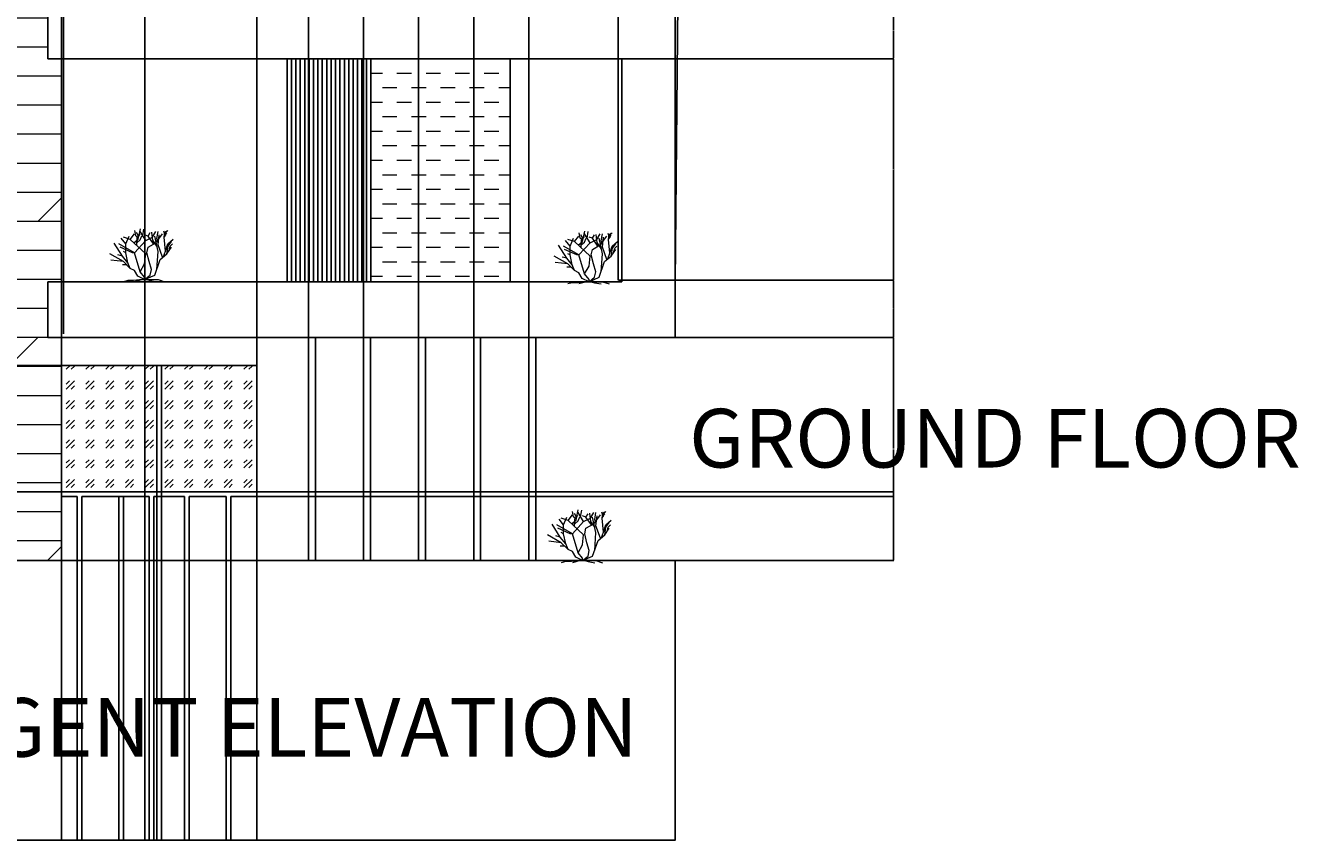
# Model space of a CAD drawing. Units: inches. Extents: x 250 to 1217, y -42 to 832.
# Tile 5 of 7: x 670 to 1217, y -42 to 309. Entities that reach past the tile are written whole.
import ezdxf

# ---------------------------------------------------------------- set-up
doc = ezdxf.new("R2010")
doc.units = ezdxf.units.IN
doc.header["$MEASUREMENT"] = 0
for name, color, linetype, lineweight in [('A-ANNO-DIMS', 2, 'Continuous', 18), ('A-ANNO-TEXT', 7, 'Continuous', 25), ('A-ELEV', 7, 'Continuous', 25), ('A-ELEV-PATT', 8, 'Continuous', 13), ('L-PLNT', 3, 'Continuous', 13)]:
    doc.layers.add(name, color=color, linetype=linetype, lineweight=lineweight)
doc.styles.get("Standard").update_dxf_attribs({"font": 'arial.ttf'})
doc.dimstyles.get("Standard").update_dxf_attribs({"dimtxt": 0.18, "dimasz": 0.18, "dimexe": 0.18, "dimexo": 0.0625, "dimgap": 0.09, "dimtad": 0, "dimtih": 1, "dimtoh": 1, "dimdec": 4, "dimzin": 0, "dimdsep": 46, "dimtxsty": 'Standard', "dimcen": 0.09, "dimadec": 0, "dimazin": 0, "dimtfac": 1, "dimtdec": 4, "dimtofl": 0, "dimtmove": 0, "dimatfit": 3, "dimfxl": 1, "dimtolj": 1, "dimtzin": 0, "dimarcsym": 0})

# ---------------------------------------------------------------- blocks, each defined once
blk = doc.blocks.new('*U2')
for p, q in [((-12.471, 19.775), (-12.898, 22.044)), ((-11.433, 18.289), (-10.457, 22.749)), ((-9.48, 19.775), (-8.992, 22.592)), ((0.041, 20.714), (1.384, 22.044)), ((-18.24, 11.04), (-21.755, 16.655)), ((-16.8, 16.32), (-18.72, 18.72)), ((-14.88, 18.24), (-17.76, 19.2)), ((-16.8, 16.32), (-15.36, 19.68)), ((-14.88, 18.24), (-12.96, 20.64)), ((-8.16, 12), (-14.88, 18.24)), ((-13.325, 16.724), (-11.433, 18.289)), ((-12.96, 12.48), (-8.16, 17.76)), ((-11.677, 19.071), (-12.471, 19.775)), ((-11.28, 19.619), (-12.104, 21.184)), ((-12.043, 15.628), (-11.921, 18.836)), ((-11.982, 16.802), (-10.579, 18.054)), ((-11.921, 18.836), (-10.64, 20.401)), ((-10.579, 18.054), (-9.846, 19.697)), ((-8.16, 17.76), (-10.56, 21.6)), ((-7.2, 19.68), (-8.64, 20.16)), ((-8.16, 17.76), (-5.28, 19.2)), ((-7.2, 19.68), (-6.24, 21.12)), ((-4.8, 16.32), (-7.2, 19.68)), ((-7.2, 14.88), (-3.84, 16.8)), ((-5.086, 17.741), (-5.513, 21.34)), ((-5.28, 19.2), (-3.84, 21.6)), ((-3.377, 15.315), (-5.086, 17.819)), ((-2.88, 12.96), (-4.32, 19.68)), ((-3.84, 16.8), (-0.96, 20.64)), ((-3.377, 18.602), (-2.888, 21.575)), ((-2.766, 16.802), (-3.377, 18.602)), ((-2.88, 15.84), (-2.4, 20.16)), ((-0.508, 21.888), (-0.081, 20.558)), ((-0.203, 19.149), (0.102, 21.34)), ((0.346, 13.203), (-0.203, 19.149)), ((-0.142, 19.384), (0.59, 20.401)), ((-0.02, 20.01), (0.896, 21.105)), ((0.102, 21.34), (0.835, 21.888)), ((1.323, 16.254), (3.642, 18.289)), ((1.44, 15.36), (2.88, 17.28)), ((-17.76, 8.64), (-23.663, 11.961)), ((-18.24, 11.04), (-20.16, 11.52)), ((-12.96, 12.48), (-19.68, 16.32)), ((-13.92, 12.48), (-19.2, 14.88)), ((-15.84, 8.16), (-18.24, 11.04)), ((-16.8, 12.48), (-17.76, 12.96)), ((-16.8, 12.48), (-16.8, 16.32)), ((-15.84, 8.16), (-16.8, 12.48)), ((-12.96, 12.48), (-13.92, 12.48)), ((-10.56, 4.32), (-12.96, 12.48)), ((-8.64, 7.68), (-8.16, 12)), ((-7.68, 12.48), (-7.2, 14.88)), ((-6.72, 8.64), (-7.68, 12.48)), ((-3.36, 5.28), (-2.88, 12.96)), ((-0.96, 10.56), (-2.88, 15.84)), ((-1.92, 9.6), (0.96, 12)), ((-0.48, 10.8), (0.346, 13.203)), ((0.346, 13.203), (1.323, 16.254)), ((0.96, 12), (1.44, 15.36)), ((0.96, 12), (2.88, 14.88)), ((1.92, 13.44), (2.4, 15.36)), ((2.4, 15.36), (3.36, 16.32)), ((-17.76, 8.64), (-23.128, 9.222)), ((-16.32, 7.2), (-18.24, 7.2)), ((-14.88, 5.76), (-17.76, 8.64)), ((-14.88, 5.76), (-15.84, 8.16)), ((-12.96, 4.8), (-14.88, 5.76)), ((-10.56, 4.32), (-8.64, 7.68)), ((-5.76, 5.28), (-6.72, 8.64)), ((-4.32, 2.88), (-1.92, 9.6)), ((-15.84, 0.48), (-17.76, 0)), ((-13.44, 0.48), (-15.84, 0.48)), ((-9.6, 0.96), (-13.44, 0.48)), ((-11.52, 2.4), (-12.96, 4.8)), ((-9.6, 0.96), (-12.96, 0)), ((-8.64, 0.96), (-11.52, 2.4)), ((-8.64, 1.92), (-10.56, 4.32)), ((-9.6, 0.96), (-7.68, 0.96)), ((-8.64, 0.96), (-4.32, 2.88)), ((-8.64, 0.96), (-6.24, 2.88)), ((-8.64, 0.96), (-8.64, 1.92)), ((-8.64, 0.96), (-2.88, 0.96)), ((-7.68, 0.96), (-6.24, 0.48)), ((-6.24, 2.88), (-5.76, 5.28)), ((-6.24, 0.48), (-3.36, 0)), ((-2.88, 0.96), (0, 0))]:
    blk.add_line(p, q)
blk = doc.blocks.new('*D7')
at = {"layer": 'A-ANNO-DIMS', "color": 0, "lineweight": -2, "transparency": 16777216}
for p, q in [((347.9, 78), (347.9, -41.6)), ((948.98, 78.86), (948.98, -41.6)), ((348.08, -41.42), (648.06, -41.42)), ((948.8, -41.42), (648.82, -41.42))]:
    blk.add_line(p, q, dxfattribs=at)
at = {"layer": 'A-ANNO-DIMS', "color": 0, "transparency": 16777216}
for points in [[(348.08, -41.39), (348.08, -41.45), (347.9, -41.42)], [(948.8, -41.39), (948.8, -41.45), (948.98, -41.42)]]:
    blk.add_solid(points, dxfattribs=at)
at = {"layer": 'Defpoints', "color": 0, "transparency": 16777216}
for p in [(347.9, 78.06), (948.98, 78.93), (948.98, -41.42)]:
    blk.add_point(p, dxfattribs=at)
at = {"layer": 'A-ANNO-DIMS', "color": 0, "transparency": 16777216, "insert": (648.44, -41.42), "char_height": 0.18, "attachment_point": 5}
blk.add_mtext('\\A1;601.1', dxfattribs=at)
blk = doc.blocks.new('*D12')
at = {"layer": 'A-ANNO-DIMS', "color": 0, "lineweight": -2, "transparency": 16777216}
for p, q in [((949.05, 174.93), (1043.08, 174.93)), ((1042.9, 174.75), (1042.9, 127.11)), ((1042.9, 79.11), (1042.9, 126.75)), ((949.05, 78.93), (1043.08, 78.93))]:
    blk.add_line(p, q, dxfattribs=at)
at = {"layer": 'A-ANNO-DIMS', "color": 0, "transparency": 16777216}
for points in [[(1042.87, 174.75), (1042.93, 174.75), (1042.9, 174.93)], [(1042.87, 79.11), (1042.93, 79.11), (1042.9, 78.93)]]:
    blk.add_solid(points, dxfattribs=at)
at = {"layer": 'Defpoints', "color": 0, "transparency": 16777216}
for p in [(948.98, 174.93), (1042.9, 174.93), (948.98, 78.93)]:
    blk.add_point(p, dxfattribs=at)
at = {"layer": 'A-ANNO-DIMS', "color": 0, "transparency": 16777216, "insert": (1042.9, 126.93), "char_height": 0.18, "attachment_point": 5}
blk.add_mtext('\\A1;96', dxfattribs=at)
blk = doc.blocks.new('*D13')
at = {"layer": 'A-ANNO-DIMS', "color": 0, "lineweight": -2, "transparency": 16777216}
for p, q in [((924.56, 199.59), (1043.08, 199.59)), ((1042.9, 199.41), (1042.9, 187.44)), ((1042.9, 175.11), (1042.9, 187.08)), ((949.05, 174.93), (1043.08, 174.93))]:
    blk.add_line(p, q, dxfattribs=at)
at = {"layer": 'A-ANNO-DIMS', "color": 0, "transparency": 16777216}
for points in [[(1042.87, 199.41), (1042.93, 199.41), (1042.9, 199.59)], [(1042.87, 175.11), (1042.93, 175.11), (1042.9, 174.93)]]:
    blk.add_solid(points, dxfattribs=at)
at = {"layer": 'Defpoints', "color": 0, "transparency": 16777216}
for p in [(924.49, 199.59), (1042.9, 199.59), (948.98, 174.93)]:
    blk.add_point(p, dxfattribs=at)
at = {"layer": 'A-ANNO-DIMS', "color": 0, "transparency": 16777216, "insert": (1042.9, 187.26), "char_height": 0.18, "attachment_point": 5}
blk.add_mtext('\\A1;24.665', dxfattribs=at)
blk = doc.blocks.new('*D14')
at = {"layer": 'A-ANNO-DIMS', "color": 0, "lineweight": -2, "transparency": 16777216}
for p, q in [((926.12, 294.93), (1043.08, 294.93)), ((1042.9, 294.75), (1042.9, 247.44)), ((1042.9, 199.77), (1042.9, 247.08)), ((924.56, 199.59), (1043.08, 199.59))]:
    blk.add_line(p, q, dxfattribs=at)
at = {"layer": 'A-ANNO-DIMS', "color": 0, "transparency": 16777216}
for points in [[(1042.87, 294.75), (1042.93, 294.75), (1042.9, 294.93)], [(1042.87, 199.77), (1042.93, 199.77), (1042.9, 199.59)]]:
    blk.add_solid(points, dxfattribs=at)
at = {"layer": 'Defpoints', "color": 0, "transparency": 16777216}
for p in [(926.06, 294.93), (1042.9, 294.93), (924.49, 199.59)]:
    blk.add_point(p, dxfattribs=at)
at = {"layer": 'A-ANNO-DIMS', "color": 0, "transparency": 16777216, "insert": (1042.9, 247.26), "char_height": 0.18, "attachment_point": 5}
blk.add_mtext('\\A1;95.34', dxfattribs=at)
blk = doc.blocks.new('*D15')
at = {"layer": 'A-ANNO-DIMS', "color": 0, "lineweight": -2, "transparency": 16777216}
for p, q in [((950.12, 318.93), (1043.08, 318.93)), ((1042.9, 318.75), (1042.9, 307.11)), ((1042.9, 295.11), (1042.9, 306.75)), ((926.12, 294.93), (1043.08, 294.93))]:
    blk.add_line(p, q, dxfattribs=at)
at = {"layer": 'A-ANNO-DIMS', "color": 0, "transparency": 16777216}
for points in [[(1042.87, 318.75), (1042.93, 318.75), (1042.9, 318.93)], [(1042.87, 295.11), (1042.93, 295.11), (1042.9, 294.93)]]:
    blk.add_solid(points, dxfattribs=at)
at = {"layer": 'Defpoints', "color": 0, "transparency": 16777216}
for p in [(950.06, 318.93), (1042.9, 318.93), (926.06, 294.93)]:
    blk.add_point(p, dxfattribs=at)
at = {"layer": 'A-ANNO-DIMS', "color": 0, "transparency": 16777216, "insert": (1042.9, 306.93), "char_height": 0.18, "attachment_point": 5}
blk.add_mtext('\\A1;24', dxfattribs=at)
blk = doc.blocks.new('*D27')
at = {"layer": 'A-ANNO-DIMS', "color": 0, "lineweight": -2, "transparency": 16777216}
for p, q in [((624.98, 174.99), (624.98, 831.77)), ((625.16, 831.59), (655.07, 831.59)), ((685.76, 831.59), (655.86, 831.59)), ((685.94, 176.49), (685.94, 831.77))]:
    blk.add_line(p, q, dxfattribs=at)
at = {"layer": 'A-ANNO-DIMS', "color": 0, "transparency": 16777216}
for points in [[(625.16, 831.62), (625.16, 831.56), (624.98, 831.59)], [(685.76, 831.62), (685.76, 831.56), (685.94, 831.59)]]:
    blk.add_solid(points, dxfattribs=at)
at = {"layer": 'Defpoints', "color": 0, "transparency": 16777216}
for p in [(685.94, 831.59), (685.94, 176.43), (624.98, 174.93)]:
    blk.add_point(p, dxfattribs=at)
at = {"layer": 'A-ANNO-DIMS', "color": 0, "transparency": 16777216, "insert": (655.46, 831.59), "char_height": 0.18, "attachment_point": 5}
blk.add_mtext('\\A1;60.96', dxfattribs=at)
blk = doc.blocks.new('*D28')
at = {"layer": 'A-ANNO-DIMS', "color": 0, "lineweight": -2, "transparency": 16777216}
for p, q in [((685.94, 176.49), (685.94, 831.77)), ((686.12, 831.59), (727.07, 831.59)), ((768.8, 831.59), (727.86, 831.59)), ((768.98, 162.99), (768.98, 831.77))]:
    blk.add_line(p, q, dxfattribs=at)
at = {"layer": 'A-ANNO-DIMS', "color": 0, "transparency": 16777216}
for points in [[(686.12, 831.62), (686.12, 831.56), (685.94, 831.59)], [(768.8, 831.62), (768.8, 831.56), (768.98, 831.59)]]:
    blk.add_solid(points, dxfattribs=at)
at = {"layer": 'Defpoints', "color": 0, "transparency": 16777216}
for p in [(768.98, 831.59), (685.94, 176.43), (768.98, 162.93)]:
    blk.add_point(p, dxfattribs=at)
at = {"layer": 'A-ANNO-DIMS', "color": 0, "transparency": 16777216, "insert": (727.46, 831.59), "char_height": 0.18, "attachment_point": 5}
blk.add_mtext('\\A1;83.04', dxfattribs=at)
blk = doc.blocks.new('*D29')
at = {"layer": 'A-ANNO-DIMS', "color": 0, "lineweight": -2, "transparency": 16777216}
for p, q in [((768.98, 162.99), (768.98, 831.77)), ((769.16, 831.59), (779.67, 831.59)), ((791.11, 831.59), (780.6, 831.59)), ((791.29, 174.99), (791.29, 831.77))]:
    blk.add_line(p, q, dxfattribs=at)
at = {"layer": 'A-ANNO-DIMS', "color": 0, "transparency": 16777216}
for points in [[(769.16, 831.62), (769.16, 831.56), (768.98, 831.59)], [(791.11, 831.62), (791.11, 831.56), (791.29, 831.59)]]:
    blk.add_solid(points, dxfattribs=at)
at = {"layer": 'Defpoints', "color": 0, "transparency": 16777216}
for p in [(791.29, 831.59), (791.29, 174.93), (768.98, 162.93)]:
    blk.add_point(p, dxfattribs=at)
at = {"layer": 'A-ANNO-DIMS', "color": 0, "transparency": 16777216, "insert": (780.13, 831.59), "char_height": 0.18, "attachment_point": 5}
blk.add_mtext('\\A1;22.303', dxfattribs=at)
blk = doc.blocks.new('*D30')
at = {"layer": 'A-ANNO-DIMS', "color": 0, "lineweight": -2, "transparency": 16777216}
for p, q in [((814.96, 174.99), (814.96, 831.77)), ((815.14, 831.59), (826.33, 831.59)), ((838.45, 831.59), (827.26, 831.59)), ((838.63, 174.99), (838.63, 831.77))]:
    blk.add_line(p, q, dxfattribs=at)
at = {"layer": 'A-ANNO-DIMS', "color": 0, "transparency": 16777216}
for points in [[(815.14, 831.62), (815.14, 831.56), (814.96, 831.59)], [(838.45, 831.62), (838.45, 831.56), (838.63, 831.59)]]:
    blk.add_solid(points, dxfattribs=at)
at = {"layer": 'Defpoints', "color": 0, "transparency": 16777216}
for p in [(838.63, 831.59), (814.96, 174.93), (838.63, 174.93)]:
    blk.add_point(p, dxfattribs=at)
at = {"layer": 'A-ANNO-DIMS', "color": 0, "transparency": 16777216, "insert": (826.8, 831.59), "char_height": 0.18, "attachment_point": 5}
blk.add_mtext('\\A1;23.674', dxfattribs=at)
blk = doc.blocks.new('*D31')
at = {"layer": 'A-ANNO-DIMS', "color": 0, "lineweight": -2, "transparency": 16777216}
for p, q in [((862.31, 174.99), (862.31, 831.77)), ((862.49, 831.59), (873.68, 831.59)), ((885.8, 831.59), (874.61, 831.59)), ((885.98, 174.99), (885.98, 831.77))]:
    blk.add_line(p, q, dxfattribs=at)
at = {"layer": 'A-ANNO-DIMS', "color": 0, "transparency": 16777216}
for points in [[(862.49, 831.62), (862.49, 831.56), (862.31, 831.59)], [(885.8, 831.62), (885.8, 831.56), (885.98, 831.59)]]:
    blk.add_solid(points, dxfattribs=at)
at = {"layer": 'Defpoints', "color": 0, "transparency": 16777216}
for p in [(885.98, 831.59), (862.31, 174.93), (885.98, 174.93)]:
    blk.add_point(p, dxfattribs=at)
at = {"layer": 'A-ANNO-DIMS', "color": 0, "transparency": 16777216, "insert": (874.15, 831.59), "char_height": 0.18, "attachment_point": 5}
blk.add_mtext('\\A1;23.674', dxfattribs=at)
blk = doc.blocks.new('*D32')
at = {"layer": 'A-ANNO-DIMS', "color": 0, "lineweight": -2, "transparency": 16777216}
for p, q in [((885.98, 174.99), (885.98, 831.77)), ((886.16, 831.59), (917.26, 831.59)), ((948.8, 831.59), (917.7, 831.59)), ((948.98, 174.99), (948.98, 831.77))]:
    blk.add_line(p, q, dxfattribs=at)
at = {"layer": 'A-ANNO-DIMS', "color": 0, "transparency": 16777216}
for points in [[(886.16, 831.62), (886.16, 831.56), (885.98, 831.59)], [(948.8, 831.62), (948.8, 831.56), (948.98, 831.59)]]:
    blk.add_solid(points, dxfattribs=at)
at = {"layer": 'Defpoints', "color": 0, "transparency": 16777216}
for p in [(948.98, 831.59), (885.98, 174.93), (948.98, 174.93)]:
    blk.add_point(p, dxfattribs=at)
at = {"layer": 'A-ANNO-DIMS', "color": 0, "transparency": 16777216, "insert": (917.48, 831.59), "char_height": 0.18, "attachment_point": 5}
blk.add_mtext('\\A1;63', dxfattribs=at)
blk = doc.blocks.new('*D36')
at = {"layer": 'A-ANNO-DIMS', "color": 0, "lineweight": -2, "transparency": 16777216}
for p, q in [((768.92, 162.93), (250.36, 162.93)), ((250.54, 162.75), (250.54, 135.88)), ((250.54, 108.65), (250.54, 135.51)), ((768.92, 108.47), (250.36, 108.47))]:
    blk.add_line(p, q, dxfattribs=at)
at = {"layer": 'A-ANNO-DIMS', "color": 0, "transparency": 16777216}
for points in [[(250.51, 162.75), (250.57, 162.75), (250.54, 162.93)], [(250.51, 108.65), (250.57, 108.65), (250.54, 108.47)]]:
    blk.add_solid(points, dxfattribs=at)
at = {"layer": 'Defpoints', "color": 0, "transparency": 16777216}
for p in [(250.54, 162.93), (768.98, 162.93), (768.98, 108.47)]:
    blk.add_point(p, dxfattribs=at)
at = {"layer": 'A-ANNO-DIMS', "color": 0, "transparency": 16777216, "insert": (250.54, 135.7), "char_height": 0.18, "attachment_point": 5}
blk.add_mtext('\\A1;54.46', dxfattribs=at)
blk = doc.blocks.new('*D52')
at = {"layer": 'A-ANNO-DIMS', "color": 0, "lineweight": -2, "transparency": 16777216}
for p, q in [((924.49, 199.65), (924.49, 831.77)), ((924.67, 831.59), (936.34, 831.59)), ((948.8, 831.59), (937.13, 831.59)), ((948.98, 198.99), (948.98, 831.77))]:
    blk.add_line(p, q, dxfattribs=at)
at = {"layer": 'A-ANNO-DIMS', "color": 0, "transparency": 16777216}
for points in [[(924.67, 831.62), (924.67, 831.56), (924.49, 831.59)], [(948.8, 831.62), (948.8, 831.56), (948.98, 831.59)]]:
    blk.add_solid(points, dxfattribs=at)
at = {"layer": 'Defpoints', "color": 0, "transparency": 16777216}
for p in [(948.98, 831.59), (924.49, 199.59), (948.98, 198.93)]:
    blk.add_point(p, dxfattribs=at)
at = {"layer": 'A-ANNO-DIMS', "color": 0, "transparency": 16777216, "insert": (936.74, 831.59), "char_height": 0.18, "attachment_point": 5}
blk.add_mtext('\\A1;24.49', dxfattribs=at)
blk = doc.blocks.new('*D65')
at = {"layer": 'A-ANNO-DIMS', "color": 0, "lineweight": -2, "transparency": 16777216}
for p, q in [((684.98, 78.86), (684.98, -41.6)), ((691.76, 78.86), (691.76, -41.6)), ((685.16, -41.42), (687.98, -41.42)), ((691.58, -41.42), (688.76, -41.42))]:
    blk.add_line(p, q, dxfattribs=at)
at = {"layer": 'A-ANNO-DIMS', "color": 0, "transparency": 16777216}
for points in [[(685.16, -41.39), (685.16, -41.45), (684.98, -41.42)], [(691.58, -41.39), (691.58, -41.45), (691.76, -41.42)]]:
    blk.add_solid(points, dxfattribs=at)
at = {"layer": 'Defpoints', "color": 0, "transparency": 16777216}
for p in [(684.98, 78.93), (691.76, 78.93), (691.76, -41.42)]:
    blk.add_point(p, dxfattribs=at)
at = {"layer": 'A-ANNO-DIMS', "color": 0, "transparency": 16777216, "insert": (688.37, -41.42), "char_height": 0.18, "attachment_point": 5}
blk.add_mtext('\\A1;6.774', dxfattribs=at)
blk = doc.blocks.new('*D66')
at = {"layer": 'A-ANNO-DIMS', "color": 0, "lineweight": -2, "transparency": 16777216}
for p, q in [((693.76, 78.86), (693.76, -41.6)), ((709.68, 78.86), (709.68, -41.6)), ((693.94, -41.42), (701.26, -41.42)), ((709.5, -41.42), (702.18, -41.42))]:
    blk.add_line(p, q, dxfattribs=at)
at = {"layer": 'A-ANNO-DIMS', "color": 0, "transparency": 16777216}
for points in [[(693.94, -41.39), (693.94, -41.45), (693.76, -41.42)], [(709.5, -41.39), (709.5, -41.45), (709.68, -41.42)]]:
    blk.add_solid(points, dxfattribs=at)
at = {"layer": 'Defpoints', "color": 0, "transparency": 16777216}
for p in [(693.76, 78.93), (709.68, 78.93), (709.68, -41.42)]:
    blk.add_point(p, dxfattribs=at)
at = {"layer": 'A-ANNO-DIMS', "color": 0, "transparency": 16777216, "insert": (701.72, -41.42), "char_height": 0.18, "attachment_point": 5}
blk.add_mtext('\\A1;15.928', dxfattribs=at)
blk = doc.blocks.new('*D67')
at = {"layer": 'A-ANNO-DIMS', "color": 0, "lineweight": -2, "transparency": 16777216}
for p, q in [((711.68, 78.86), (711.68, -41.6)), ((722.76, 78.86), (722.76, -41.6)), ((711.86, -41.42), (716.77, -41.42)), ((722.58, -41.42), (717.67, -41.42))]:
    blk.add_line(p, q, dxfattribs=at)
at = {"layer": 'A-ANNO-DIMS', "color": 0, "transparency": 16777216}
for points in [[(711.86, -41.39), (711.86, -41.45), (711.68, -41.42)], [(722.58, -41.39), (722.58, -41.45), (722.76, -41.42)]]:
    blk.add_solid(points, dxfattribs=at)
at = {"layer": 'Defpoints', "color": 0, "transparency": 16777216}
for p in [(711.68, 78.93), (722.76, 78.93), (722.76, -41.42)]:
    blk.add_point(p, dxfattribs=at)
at = {"layer": 'A-ANNO-DIMS', "color": 0, "transparency": 16777216, "insert": (717.22, -41.42), "char_height": 0.18, "attachment_point": 5}
blk.add_mtext('\\A1;11.072', dxfattribs=at)
blk = doc.blocks.new('*D68')
at = {"layer": 'A-ANNO-DIMS', "color": 0, "lineweight": -2, "transparency": 16777216}
for p, q in [((724.76, 78.86), (724.76, -41.6)), ((737.98, 78.86), (737.98, -41.6)), ((724.94, -41.42), (730.91, -41.42)), ((737.8, -41.42), (731.82, -41.42))]:
    blk.add_line(p, q, dxfattribs=at)
at = {"layer": 'A-ANNO-DIMS', "color": 0, "transparency": 16777216}
for points in [[(724.94, -41.39), (724.94, -41.45), (724.76, -41.42)], [(737.8, -41.39), (737.8, -41.45), (737.98, -41.42)]]:
    blk.add_solid(points, dxfattribs=at)
at = {"layer": 'Defpoints', "color": 0, "transparency": 16777216}
for p in [(724.76, 78.93), (737.98, 78.93), (737.98, -41.42)]:
    blk.add_point(p, dxfattribs=at)
at = {"layer": 'A-ANNO-DIMS', "color": 0, "transparency": 16777216, "insert": (731.37, -41.42), "char_height": 0.18, "attachment_point": 5}
blk.add_mtext('\\A1;13.226', dxfattribs=at)
blk = doc.blocks.new('*D69')
at = {"layer": 'A-ANNO-DIMS', "color": 0, "lineweight": -2, "transparency": 16777216}
for p, q in [((739.98, 78.86), (739.98, -41.6)), ((755.91, 78.86), (755.91, -41.6)), ((740.16, -41.42), (747.49, -41.42)), ((755.73, -41.42), (748.4, -41.42))]:
    blk.add_line(p, q, dxfattribs=at)
at = {"layer": 'A-ANNO-DIMS', "color": 0, "transparency": 16777216}
for points in [[(740.16, -41.39), (740.16, -41.45), (739.98, -41.42)], [(755.73, -41.39), (755.73, -41.45), (755.91, -41.42)]]:
    blk.add_solid(points, dxfattribs=at)
at = {"layer": 'Defpoints', "color": 0, "transparency": 16777216}
for p in [(739.98, 78.93), (755.91, 78.93), (755.91, -41.42)]:
    blk.add_point(p, dxfattribs=at)
at = {"layer": 'A-ANNO-DIMS', "color": 0, "transparency": 16777216, "insert": (747.95, -41.42), "char_height": 0.18, "attachment_point": 5}
blk.add_mtext('\\A1;15.928', dxfattribs=at)
blk = doc.blocks.new('*D70')
at = {"layer": 'A-ANNO-DIMS', "color": 0, "lineweight": -2, "transparency": 16777216}
for p, q in [((757.91, 78.86), (757.91, -41.6)), ((768.98, 78.86), (768.98, -41.6)), ((758.09, -41.42), (762.99, -41.42)), ((768.8, -41.42), (763.9, -41.42))]:
    blk.add_line(p, q, dxfattribs=at)
at = {"layer": 'A-ANNO-DIMS', "color": 0, "transparency": 16777216}
for points in [[(758.09, -41.39), (758.09, -41.45), (757.91, -41.42)], [(768.8, -41.39), (768.8, -41.45), (768.98, -41.42)]]:
    blk.add_solid(points, dxfattribs=at)
at = {"layer": 'Defpoints', "color": 0, "transparency": 16777216}
for p in [(757.91, 78.93), (768.98, 78.93), (768.98, -41.42)]:
    blk.add_point(p, dxfattribs=at)
at = {"layer": 'A-ANNO-DIMS', "color": 0, "transparency": 16777216, "insert": (763.45, -41.42), "char_height": 0.18, "attachment_point": 5}
blk.add_mtext('\\A1;11.072', dxfattribs=at)
blk = doc.blocks.new('*D75')
at = {"layer": 'A-ANNO-DIMS', "color": 0, "lineweight": -2, "transparency": 16777216}
for p, q in [((684.98, 108.4), (684.98, -41.6)), ((725.98, 108.4), (725.98, -41.6)), ((685.16, -41.42), (705.09, -41.42)), ((725.8, -41.42), (705.88, -41.42))]:
    blk.add_line(p, q, dxfattribs=at)
at = {"layer": 'A-ANNO-DIMS', "color": 0, "transparency": 16777216}
for points in [[(685.16, -41.39), (685.16, -41.45), (684.98, -41.42)], [(725.8, -41.39), (725.8, -41.45), (725.98, -41.42)]]:
    blk.add_solid(points, dxfattribs=at)
at = {"layer": 'Defpoints', "color": 0, "transparency": 16777216}
for p in [(684.98, 108.47), (725.98, 108.47), (725.98, -41.42)]:
    blk.add_point(p, dxfattribs=at)
at = {"layer": 'A-ANNO-DIMS', "color": 0, "transparency": 16777216, "insert": (705.48, -41.42), "char_height": 0.18, "attachment_point": 5}
blk.add_mtext('\\A1;41.00', dxfattribs=at)
blk = doc.blocks.new('*D76')
at = {"layer": 'A-ANNO-DIMS', "color": 0, "lineweight": -2, "transparency": 16777216}
for p, q in [((727.98, 108.4), (727.98, -41.6)), ((768.98, 108.4), (768.98, -41.6)), ((728.16, -41.42), (748.09, -41.42)), ((768.8, -41.42), (748.88, -41.42))]:
    blk.add_line(p, q, dxfattribs=at)
at = {"layer": 'A-ANNO-DIMS', "color": 0, "transparency": 16777216}
for points in [[(728.16, -41.39), (728.16, -41.45), (727.98, -41.42)], [(768.8, -41.39), (768.8, -41.45), (768.98, -41.42)]]:
    blk.add_solid(points, dxfattribs=at)
at = {"layer": 'Defpoints', "color": 0, "transparency": 16777216}
for p in [(727.98, 108.47), (768.98, 108.47), (768.98, -41.42)]:
    blk.add_point(p, dxfattribs=at)
at = {"layer": 'A-ANNO-DIMS', "color": 0, "transparency": 16777216, "insert": (748.48, -41.42), "char_height": 0.18, "attachment_point": 5}
blk.add_mtext('\\A1;41.00', dxfattribs=at)
blk = doc.blocks.new('*D77')
at = {"layer": 'A-ANNO-DIMS', "color": 0, "lineweight": -2, "transparency": 16777216}
for p, q in [((769.05, 108.47), (1043.08, 108.47)), ((769.05, 106.47), (1043.08, 106.47)), ((1042.9, 108.29), (1042.9, 107.65)), ((1042.9, 106.65), (1042.9, 107.28))]:
    blk.add_line(p, q, dxfattribs=at)
at = {"layer": 'A-ANNO-DIMS', "color": 0, "transparency": 16777216}
for points in [[(1042.87, 108.29), (1042.93, 108.29), (1042.9, 108.47)], [(1042.87, 106.65), (1042.93, 106.65), (1042.9, 106.47)]]:
    blk.add_solid(points, dxfattribs=at)
at = {"layer": 'Defpoints', "color": 0, "transparency": 16777216}
for p in [(768.98, 108.47), (768.98, 106.47), (1042.9, 108.47)]:
    blk.add_point(p, dxfattribs=at)
at = {"layer": 'A-ANNO-DIMS', "color": 0, "transparency": 16777216, "insert": (1042.9, 107.47), "char_height": 0.18, "attachment_point": 5}
blk.add_mtext('\\A1;2.00', dxfattribs=at)
blk = doc.blocks.new('*D98')
at = {"layer": 'A-ANNO-DIMS', "color": 0, "lineweight": -2, "transparency": 16777216}
for p, q in [((685.06, 582.86), (685.06, -41.6)), ((720.87, 583.82), (720.87, -41.6)), ((685.24, -41.42), (702.59, -41.42)), ((720.69, -41.42), (703.34, -41.42))]:
    blk.add_line(p, q, dxfattribs=at)
at = {"layer": 'A-ANNO-DIMS', "color": 0, "transparency": 16777216}
for points in [[(685.24, -41.39), (685.24, -41.45), (685.06, -41.42)], [(720.69, -41.39), (720.69, -41.45), (720.87, -41.42)]]:
    blk.add_solid(points, dxfattribs=at)
at = {"layer": 'Defpoints', "color": 0, "transparency": 16777216}
for p in [(685.06, 582.93), (720.87, 583.89), (720.87, -41.42)]:
    blk.add_point(p, dxfattribs=at)
at = {"layer": 'A-ANNO-DIMS', "color": 0, "transparency": 16777216, "insert": (702.97, -41.42), "char_height": 0.18, "attachment_point": 5}
blk.add_mtext('\\A1;35.81', dxfattribs=at)

msp = doc.modelspace()

# ---------------------------------------------------------------- hatches: boundary and pattern name
at = {"layer": 'A-ELEV-PATT'}
h = msp.add_hatch(dxfattribs=at)
h.set_pattern_fill('DOLMIT', color=256, scale=50)
h.paths.add_polyline_path([(684.9826, 558.9271), (679.1872, 558.9271), (679.1872, 582.9271), (685.0649, 582.9271), (685.0649, 678.9271), (679.1872, 678.9271), (679.1872, 702.9271), (630.7779, 702.9271), (630.7779, 678.9271), (625.0649, 678.9271), (625.0649, 582.9271), (630.7779, 582.9271), (630.7779, 558.9271), (624.9826, 558.9271), (624.9826, 438.9271), (630.7779, 438.9271), (630.7779, 414.9271), (624.9826, 414.9271), (624.9826, 318.9271), (630.7779, 318.9271), (630.7779, 294.9271), (624.9826, 294.9271), (624.9826, 198.9271), (630.7779, 198.9271), (630.7779, 174.9271), (624.9826, 174.9271), (624.9826, 78.9271), (684.9826, 78.9271), (684.9826, 174.9271), (679.1872, 174.9271), (679.1872, 198.9271), (683.6004, 198.9271), (684.9826, 198.9271), (684.9826, 294.9271), (679.1872, 294.9271), (679.1872, 318.9271), (684.9826, 318.9271), (684.9826, 414.9271), (679.1872, 414.9271), (679.1872, 438.9271), (684.9826, 438.9271)])
h = msp.add_hatch(dxfattribs=at)
h.set_pattern_fill('DASH', color=256, scale=50)
h.set_pattern_definition([(0, (373.068, 120), (6.25, 6.25), [6.25, -6.25])])
h.paths.add_polyline_path([(878.0509, 294.9271), (818.0509, 294.9271), (818.0509, 198.9271), (878.0509, 198.9271)])
h = msp.add_hatch(dxfattribs=at)
h.set_pattern_fill('GOST_GLASS', color=256)
h.set_pattern_definition([(45, (144, 2e-13), (8.48528, 0), [5, -7]), (45, (146.1213, 2e-13), (8.48528, 0), [2, -10]), (45, (144, 2.1213), (8.48528, 0), [2, -10])])
h.paths.add_polyline_path([(725.9826, 162.9271), (684.9826, 162.9271), (684.9826, 108.4651), (722.7563, 108.4651), (725.9826, 108.4651)])
h.paths.add_polyline_path([(768.9826, 162.9271), (727.9826, 162.9271), (727.9826, 108.4651), (768.9826, 108.4651)])

# ---------------------------------------------------------------- linework, layer by layer
at = {"layer": 'A-ELEV'}
for p, q in [((679.1872, 318.9271), (679.1872, 294.9271)), ((684.9826, 294.9271), (684.9826, 198.9271)), ((782.0509, 294.9271), (782.0509, 198.9271)), ((783.9456, 294.9271), (783.9456, 198.9271)), ((785.8403, 294.9271), (785.8403, 198.9271)), ((787.7351, 294.9271), (787.7351, 198.9271)), ((789.6298, 294.9271), (789.6298, 198.9271)), ((791.5246, 294.9271), (791.5246, 198.9271)), ((793.4193, 294.9271), (793.4193, 198.9271)), ((795.314, 294.9271), (795.314, 198.9271)), ((797.2088, 294.9271), (797.2088, 198.9271)), ((799.1035, 294.9271), (799.1035, 198.9271)), ((800.9982, 294.9271), (800.9982, 198.9271)), ((802.893, 294.9271), (802.893, 198.9271)), ((804.7877, 294.9271), (804.7877, 198.9271)), ((806.6824, 294.9271), (806.6824, 198.9271)), ((808.5772, 294.9271), (808.5772, 198.9271)), ((810.4719, 294.9271), (810.4719, 198.9271)), ((812.3667, 294.9271), (812.3667, 198.9271)), ((814.2614, 294.9271), (814.2614, 198.9271)), ((816.1561, 294.9271), (816.1561, 198.9271)), ((818.0509, 294.9271), (818.0509, 198.9271)), ((818.0509, 294.9271), (818.0509, 198.9271)), ((818.0509, 294.9271), (818.0509, 198.9271)), ((818.0509, 294.9271), (818.0509, 198.9271)), ((878.0509, 294.9271), (878.0509, 198.9271)), ((926.0561, 198.9271), (679.1872, 198.9271)), ((683.6004, 198.9271), (679.1872, 198.9271)), ((679.1872, 198.9271), (679.1872, 174.9271)), ((679.1872, 198.9271), (926.0561, 198.9271)), ((948.9826, 174.9271), (948.9826, 198.9271)), ((948.9826, 174.9271), (679.1872, 174.9271)), ((684.9826, 174.9271), (684.9826, 78.9271)), ((791.2851, 174.9271), (791.2851, 78.9271)), ((794.2851, 174.9271), (794.2851, 78.9271)), ((814.9595, 174.9271), (814.9595, 78.9271)), ((817.9595, 174.9271), (817.9595, 78.9271)), ((838.6339, 174.9271), (838.6339, 78.9271)), ((841.6339, 174.9271), (841.6339, 78.9271)), ((862.3082, 174.9271), (862.3082, 78.9271)), ((865.3082, 174.9271), (865.3082, 78.9271)), ((885.9826, 174.9271), (885.9826, 78.9271)), ((888.9826, 174.9271), (888.9826, 78.9271)), ((684.9826, 162.9271), (768.9826, 162.9271)), ((725.9826, 162.9271), (725.9826, 108.4651)), ((727.9826, 162.9271), (727.9826, 108.4651)), ((768.9826, 162.9271), (768.9826, 78.9271)), ((722.7563, 108.4651), (684.9826, 108.4651)), ((691.7563, 106.4651), (684.9826, 106.4651)), ((691.7563, 106.4651), (691.7563, 78.9271)), ((693.7563, 106.4651), (693.7563, 78.9271)), ((709.684, 106.4651), (693.7563, 106.4651)), ((768.9826, 108.4651), (708.9826, 108.4651)), ((722.7563, 106.4651), (708.9826, 106.4651)), ((709.684, 106.4651), (709.684, 78.9271)), ((722.7563, 106.4651), (711.684, 106.4651)), ((711.684, 106.4651), (711.684, 78.9271)), ((722.7563, 106.4651), (722.7563, 78.9271)), ((737.9826, 106.4651), (724.7563, 106.4651)), ((724.7563, 106.4651), (724.7563, 78.9271)), ((737.9826, 106.4651), (737.9826, 78.9271)), ((739.9826, 106.4651), (739.9826, 78.9271)), ((755.9103, 106.4651), (739.9826, 106.4651)), ((755.9103, 106.4651), (755.9103, 78.9271)), ((768.9826, 106.4651), (757.9103, 106.4651)), ((757.9103, 106.4651), (757.9103, 78.9271)), ((348.9826, 78.9271), (948.9826, 78.9271))]:
    msp.add_line(p, q, dxfattribs=at)
for points in [[(948.9826, 198.9271), (950.0561, 318.9271), (679.1872, 318.9271)], [(926.0561, 198.9271), (926.0561, 294.9271), (679.1872, 294.9271)]]:
    msp.add_lwpolyline(points, dxfattribs=at)

# ---------------------------------------------------------------- block references
at = {"layer": 'L-PLNT'}
for p in [(729.43, 198.9271), (920.5513, 197.9671), (917.7694, 77.9671)]:
    msp.add_blockref('*U2', p, dxfattribs=at)

# ---------------------------------------------------------------- texts
at = {"layer": 'A-ANNO-TEXT'}
for s, p in [('GROUND FLOOR', (954.9807, 118.9625)), ('G+4 ELEGENT ELEVATION ', (525.3922, -5.5103))]:
    msp.add_text(s, height=25.254387, dxfattribs=at).set_placement(p)

# ---------------------------------------------------------------- dimensions: what is measured, and where the dimension line sits
at = {"layer": 'A-ANNO-DIMS'}
for base, p1, p2, override, picture, middle in [((685.944, 831.5941), (624.9826, 174.9271), (685.944, 176.4321), {"dimdec": 2, "dimlfac": 1, "dimrnd": 0, "dimzin": 0, "dimdsep": 46, "dimlunit": 2}, '*D27', (655.4633, 831.5941)), ((768.9826, 831.5941), (685.944, 176.4321), (768.9826, 162.9271), {"dimdec": 2, "dimlfac": 1, "dimrnd": 0, "dimzin": 0, "dimdsep": 46, "dimlunit": 2}, '*D28', (727.4633, 831.5941)), ((791.28513, 831.59407), (768.98257, 162.92707), (791.28513, 174.92707), {"dimdec": 3, "dimlfac": 1, "dimrnd": 0, "dimzin": 0, "dimdsep": 46, "dimlunit": 2}, '*D29', (780.13385, 831.59407)), ((838.6339, 831.5941), (814.9595, 174.9271), (838.6339, 174.9271), {"dimdec": 3, "dimlfac": 1, "dimrnd": 0, "dimzin": 0, "dimdsep": 46, "dimlunit": 2}, '*D30', (826.7967, 831.5941)), ((885.9826, 831.5941), (862.3082, 174.9271), (885.9826, 174.9271), {"dimdec": 3, "dimlfac": 1, "dimrnd": 0, "dimzin": 0, "dimdsep": 46, "dimlunit": 2}, '*D31', (874.1454, 831.5941)), ((948.9826, 831.5941), (885.9826, 174.9271), (948.9826, 174.9271), {"dimdec": 0, "dimlfac": 1, "dimrnd": 0, "dimzin": 0, "dimdsep": 46, "dimlunit": 2}, '*D32', (917.4826, 831.5941)), ((948.9826, 831.5941), (924.4933, 199.5921), (948.9826, 198.9271), {"dimdec": 2, "dimlfac": 1, "dimrnd": 0, "dimzin": 0, "dimdsep": 46, "dimlunit": 2}, '*D52', (936.7379, 831.5941)), ((720.8723, -41.4199), (685.0649, 582.9271), (720.8723, 583.8871), {"dimdec": 2, "dimlfac": 1, "dimrnd": 0, "dimzin": 0, "dimdsep": 46, "dimlunit": 2}, '*D98', (702.9686, -41.4199)), ((725.9826, -41.4199), (684.9826, 108.4651), (725.9826, 108.4651), {"dimdec": 2, "dimlfac": 1, "dimrnd": 0, "dimzin": 0, "dimdsep": 46, "dimlunit": 2}, '*D75', (705.4826, -41.4199)), ((768.9826, -41.4199), (727.9826, 108.4651), (768.9826, 108.4651), {"dimdec": 2, "dimlfac": 1, "dimrnd": 0, "dimzin": 0, "dimdsep": 46, "dimlunit": 2}, '*D76', (748.4826, -41.4199)), ((948.9826, -41.4199), (347.8976, 78.0612), (948.9826, 78.9271), {"dimdec": 1, "dimlfac": 1, "dimrnd": 0, "dimzin": 0, "dimdsep": 46, "dimlunit": 2}, '*D7', (648.4401, -41.4199)), ((691.7563, -41.4199), (684.9826, 78.9271), (691.7563, 78.9271), {"dimdec": 3, "dimlfac": 1, "dimrnd": 0, "dimzin": 0, "dimdsep": 46, "dimlunit": 2}, '*D65', (688.3694, -41.4199)), ((709.684, -41.4199), (693.7563, 78.9271), (709.684, 78.9271), {"dimdec": 3, "dimlfac": 1, "dimrnd": 0, "dimzin": 0, "dimdsep": 46, "dimlunit": 2}, '*D66', (701.7201, -41.4199)), ((722.7563, -41.4199), (711.684, 78.9271), (722.7563, 78.9271), {"dimdec": 3, "dimlfac": 1, "dimrnd": 0, "dimzin": 0, "dimdsep": 46, "dimlunit": 2}, '*D67', (717.2201, -41.4199)), ((737.9826, -41.4199), (724.7563, 78.9271), (737.9826, 78.9271), {"dimdec": 3, "dimlfac": 1, "dimrnd": 0, "dimzin": 0, "dimdsep": 46, "dimlunit": 2}, '*D68', (731.3694, -41.4199)), ((755.9103, -41.4199), (739.9826, 78.9271), (755.9103, 78.9271), {"dimdec": 3, "dimlfac": 1, "dimrnd": 0, "dimzin": 0, "dimdsep": 46, "dimlunit": 2}, '*D69', (747.9464, -41.4199)), ((768.9826, -41.4199), (757.9103, 78.9271), (768.9826, 78.9271), {"dimdec": 3, "dimlfac": 1, "dimrnd": 0, "dimzin": 0, "dimdsep": 46, "dimlunit": 2}, '*D70', (763.4464, -41.4199))]:
    dim = msp.add_linear_dim(base=base, p1=p1, p2=p2, dimstyle='Standard', override=override, dxfattribs=at)
    dim.commit()
    dim.dimension.update_dxf_attribs({"geometry": picture, "text_midpoint": middle})
for base, p1, p2, override, picture, middle in [((1042.8996, 318.9271), (926.0561, 294.9271), (950.0561, 318.9271), {"dimdec": 0, "dimlfac": 1, "dimrnd": 0, "dimzin": 0, "dimdsep": 46, "dimlunit": 2}, '*D15', (1042.8996, 306.9271)), ((1042.899582, 294.927068), (924.493263, 199.592068), (926.056094, 294.927068), {"dimdec": 2, "dimlfac": 1, "dimrnd": 0, "dimzin": 0, "dimdsep": 46, "dimlunit": 2}, '*D14', (1042.899582, 247.259568)), ((1042.8996, 199.5921), (948.9826, 174.9271), (924.4933, 199.5921), {"dimdec": 3, "dimlfac": 1, "dimrnd": 0, "dimzin": 0, "dimdsep": 46, "dimlunit": 2}, '*D13', (1042.8996, 187.2596)), ((1042.8996, 174.9271), (948.9826, 78.9271), (948.9826, 174.9271), {"dimdec": 0, "dimlfac": 1, "dimrnd": 0, "dimzin": 0, "dimdsep": 46, "dimlunit": 2}, '*D12', (1042.8996, 126.9271)), ((250.5369, 162.9271), (768.9826, 108.4651), (768.9826, 162.9271), {"dimdec": 2, "dimlfac": 1, "dimrnd": 0, "dimzin": 0, "dimdsep": 46, "dimlunit": 2}, '*D36', (250.5369, 135.6961)), ((1042.8996, 108.4651), (768.9826, 106.4651), (768.9826, 108.4651), {"dimdec": 2, "dimlfac": 1, "dimrnd": 0, "dimzin": 0, "dimdsep": 46, "dimlunit": 2}, '*D77', (1042.8996, 107.4651))]:
    dim = msp.add_linear_dim(base=base, p1=p1, p2=p2, angle=90, dimstyle='Standard', override=override, dxfattribs=at)
    dim.commit()
    dim.dimension.update_dxf_attribs({"geometry": picture, "text_midpoint": middle})

doc.saveas('drawing.dxf')
